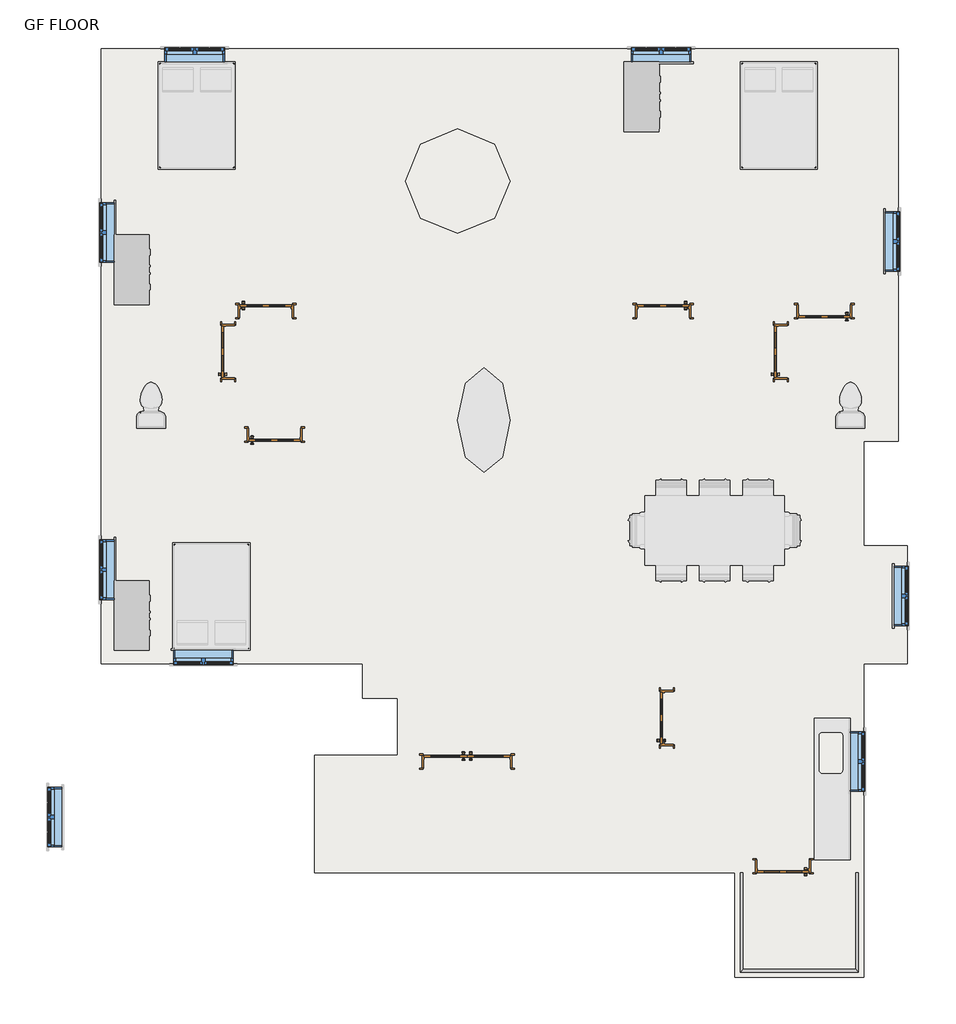
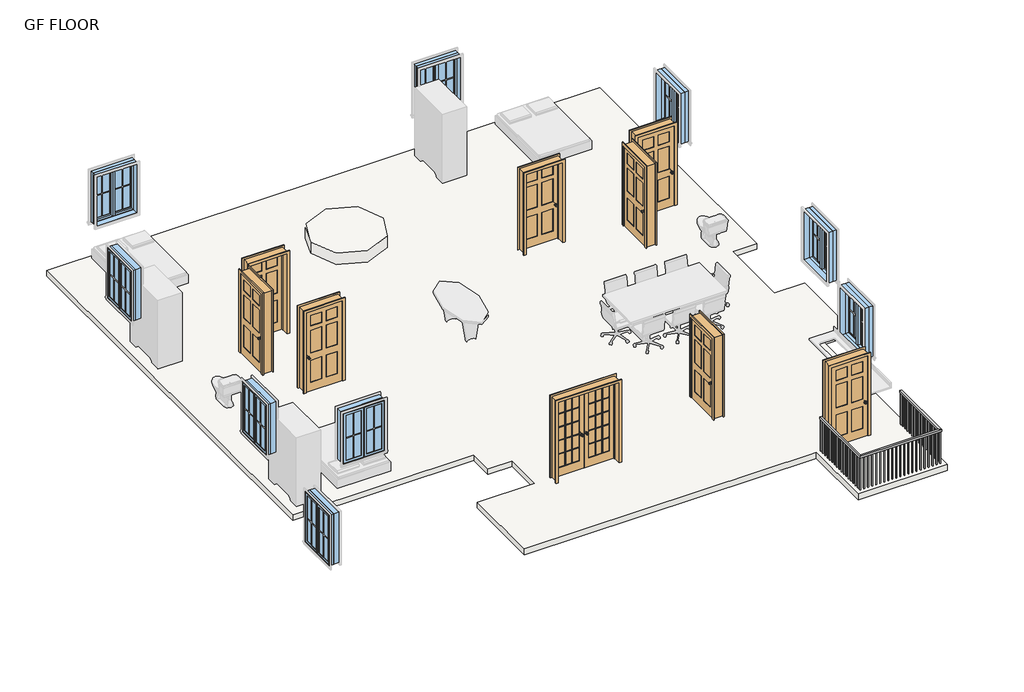
# One storey, part 1 of 2: 9 doors, 9 windows, 2 slabs, 1 railing.
"""IFC4 building model written with IfcOpenShell, lengths in millimetres."""

from ifc_helpers import new_model, si_unit, point, frame, frame_2d, origin, place, context, project, spatial, polyline, circle_curve, trimmed, segment, composite_curve, outline, extrude, faceted_brep, transform, mapped, element, save
from components import door_610bc5f6, door_d86b6c54, door_c5239341, window_c95ebb39

model = new_model("IFC4")

# Units and contexts
model_context = context("Model", 3, world=origin())
ifc_project = project(units=[si_unit("LENGTHUNIT", "METRE", prefix="MILLI")], contexts=[model_context])

# Site, building, storey
site = spatial("IfcSite", under=ifc_project)
building = spatial("IfcBuilding", under=site)
storey = spatial("IfcBuildingStorey", under=building, Name="GF FLOOR", Elevation=914.4)

# Doors
placement = place(None, origin())
door_shape = door_610bc5f6(model_context)
element("IfcDoor", 1, ObjectType="Door-Interior-Double-Full Glass-Wood : 60\" x 84\"", at=placement, inside=storey, context=model_context, shape_type="MappedRepresentation", body=[
    mapped(door_shape, transform((4931.2512825, 2078.7656886, 914.4), x_axis=(1.0, 0.0, 0.0), y_axis=(0.0, 1.0, 0.0), z_axis=(0.0, 0.0, 1.0))),
])
door_2_shape = door_d86b6c54(model_context)
element("IfcDoor", 2, ObjectType="Door-Interior-Single-6_Panel-Wood : 36\" x 84\"", at=placement, inside=storey, context=model_context, shape_type="MappedRepresentation", body=[
    mapped(door_2_shape, transform((8420.5762825, 2837.5906886, 914.4), x_axis=(0.0, 1.0, 0.0), y_axis=(-1.0, 0.0, 0.0), z_axis=(0.0, 0.0, 1.0))),
])
element("IfcDoor", 3, ObjectType="Door-Interior-Single-6_Panel-Wood : 36\" x 84\"", at=placement, inside=storey, context=model_context, shape_type="MappedRepresentation", body=[
    mapped(door_2_shape, transform((10455.7512825, 243.6156886, 914.4), x_axis=(-1.0, 0.0, 0.0), y_axis=(0.0, -1.0, 0.0), z_axis=(0.0, 0.0, 1.0))),
])
element("IfcDoor", 4, ObjectType="Door-Interior-Single-6_Panel-Wood : 36\" x 84\"", at=placement, inside=storey, context=model_context, shape_type="MappedRepresentation", body=[
    mapped(door_2_shape, transform((11179.6512825, 9946.4156886, 914.4), x_axis=(-1.0, 0.0, 0.0), y_axis=(0.0, -1.0, 0.0), z_axis=(0.0, 0.0, 1.0))),
])
element("IfcDoor", 5, ObjectType="Door-Interior-Single-6_Panel-Wood : 36\" x 84\"", at=placement, inside=storey, context=model_context, shape_type="MappedRepresentation", body=[
    mapped(door_2_shape, transform((749.7762825, 9238.3906886, 914.4), x_axis=(0.0, 1.0, 0.0), y_axis=(-1.0, 0.0, 0.0), z_axis=(0.0, 0.0, 1.0))),
])
element("IfcDoor", 6, ObjectType="Door-Interior-Single-6_Panel-Wood : 36\" x 84\"", at=placement, inside=storey, context=model_context, shape_type="MappedRepresentation", body=[
    mapped(door_2_shape, transform((1413.3512825, 9952.7656886, 914.4), x_axis=(1.0, 0.0, 0.0), y_axis=(0.0, 1.0, 0.0), z_axis=(0.0, 0.0, 1.0))),
])
element("IfcDoor", 7, ObjectType="Door-Interior-Single-6_Panel-Wood : 36\" x 84\"", at=placement, inside=storey, context=model_context, shape_type="MappedRepresentation", body=[
    mapped(door_2_shape, transform((10414.4762825, 9238.3906886, 914.4), x_axis=(0.0, 1.0, 0.0), y_axis=(-1.0, 0.0, 0.0), z_axis=(0.0, 0.0, 1.0))),
])
door_3_shape = door_c5239341(model_context)
element("IfcDoor", 8, ObjectType="Door-Interior-Single-6_Panel-Wood : 36\" x 84\"", at=placement, inside=storey, context=model_context, shape_type="MappedRepresentation", body=[
    mapped(door_3_shape, transform((1565.7512825, 7787.4156886, 914.4), x_axis=(1.0, 0.0, 0.0), y_axis=(0.0, 1.0, 0.0), z_axis=(0.0, 0.0, 1.0))),
])
element("IfcDoor", 9, ObjectType="Door-Interior-Single-6_Panel-Wood : 36\" x 84\"", at=placement, inside=storey, context=model_context, shape_type="MappedRepresentation", body=[
    mapped(door_3_shape, transform((8360.2512825, 9952.7656886, 914.4), x_axis=(-1.0, 0.0, 0.0), y_axis=(0.0, -1.0, 0.0), z_axis=(0.0, 0.0, 1.0))),
])

# Railing
element("IfcRailing", 10, ObjectType="Handrail - Rectangular", at=placement, inside=storey, context=model_context, shape_type="SolidModel", body=[
    faceted_brep([(9757.2512825, 132.4906886, 1828.8), (9757.2512825, 132.4906886, 1778.0), (9706.4512825, 132.4906886, 1778.0), (9706.4512825, 132.4906886, 1828.8), (9757.2512825, -1556.6093114, 1828.8), (9757.2512825, -1556.6093114, 1778.0), (9706.4512825, -1607.4093114, 1778.0), (9706.4512825, -1607.4093114, 1828.8), (11725.7512825, -1556.6093114, 1828.8), (11725.7512825, -1556.6093114, 1778.0), (11776.5512825, -1607.4093114, 1778.0), (11776.5512825, -1607.4093114, 1828.8), (11725.7512825, 132.4906886, 1828.8), (11776.5512825, 132.4906886, 1828.8), (11776.5512825, 132.4906886, 1778.0), (11725.7512825, 132.4906886, 1778.0)], [[[0, 1, 2, 3]], [[1, 0, 4, 5]], [[2, 1, 5, 6]], [[3, 2, 6, 7]], [[0, 3, 7, 4]], [[5, 4, 8, 9]], [[6, 5, 9, 10]], [[7, 6, 10, 11]], [[4, 7, 11, 8]], [[12, 13, 14, 15]], [[9, 8, 12, 15]], [[10, 9, 15, 14]], [[11, 10, 14, 13]], [[8, 11, 13, 12]]]),
    extrude(outline(polyline([(11760.6762825, 34.0656886), (11741.6262825, 34.0656886), (11741.6262825, 53.1156886), (11760.6762825, 53.1156886), (11760.6762825, 34.0656886)])), frame((0.0, 0.0, 914.4), z_axis=(0.0, 0.0, 1.0), x_axis=(1.0, 0.0, 0.0)), (0.0, 0.0, 1.0), 863.6),
    extrude(outline(polyline([(11760.6762825, -67.5343114), (11741.6262825, -67.5343114), (11741.6262825, -48.4843114), (11760.6762825, -48.4843114), (11760.6762825, -67.5343114)])), frame((0.0, 0.0, 914.4), z_axis=(0.0, 0.0, 1.0), x_axis=(1.0, 0.0, 0.0)), (0.0, 0.0, 1.0), 863.6),
    extrude(outline(polyline([(11760.6762825, -169.1343114), (11741.6262825, -169.1343114), (11741.6262825, -150.0843114), (11760.6762825, -150.0843114), (11760.6762825, -169.1343114)])), frame((0.0, 0.0, 914.4), z_axis=(0.0, 0.0, 1.0), x_axis=(1.0, 0.0, 0.0)), (0.0, 0.0, 1.0), 863.6),
    extrude(outline(polyline([(11760.6762825, -270.7343114), (11741.6262825, -270.7343114), (11741.6262825, -251.6843114), (11760.6762825, -251.6843114), (11760.6762825, -270.7343114)])), frame((0.0, 0.0, 914.4), z_axis=(0.0, 0.0, 1.0), x_axis=(1.0, 0.0, 0.0)), (0.0, 0.0, 1.0), 863.6),
    extrude(outline(polyline([(11760.6762825, -372.3343114), (11741.6262825, -372.3343114), (11741.6262825, -353.2843114), (11760.6762825, -353.2843114), (11760.6762825, -372.3343114)])), frame((0.0, 0.0, 914.4), z_axis=(0.0, 0.0, 1.0), x_axis=(1.0, 0.0, 0.0)), (0.0, 0.0, 1.0), 863.6),
    extrude(outline(polyline([(11760.6762825, -473.9343114), (11741.6262825, -473.9343114), (11741.6262825, -454.8843114), (11760.6762825, -454.8843114), (11760.6762825, -473.9343114)])), frame((0.0, 0.0, 914.4), z_axis=(0.0, 0.0, 1.0), x_axis=(1.0, 0.0, 0.0)), (0.0, 0.0, 1.0), 863.6),
    extrude(outline(polyline([(11760.6762825, -575.5343114), (11741.6262825, -575.5343114), (11741.6262825, -556.4843114), (11760.6762825, -556.4843114), (11760.6762825, -575.5343114)])), frame((0.0, 0.0, 914.4), z_axis=(0.0, 0.0, 1.0), x_axis=(1.0, 0.0, 0.0)), (0.0, 0.0, 1.0), 863.6),
    extrude(outline(polyline([(11760.6762825, -677.1343114), (11741.6262825, -677.1343114), (11741.6262825, -658.0843114), (11760.6762825, -658.0843114), (11760.6762825, -677.1343114)])), frame((0.0, 0.0, 914.4), z_axis=(0.0, 0.0, 1.0), x_axis=(1.0, 0.0, 0.0)), (0.0, 0.0, 1.0), 863.6),
    extrude(outline(polyline([(11760.6762825, -778.7343114), (11741.6262825, -778.7343114), (11741.6262825, -759.6843114), (11760.6762825, -759.6843114), (11760.6762825, -778.7343114)])), frame((0.0, 0.0, 914.4), z_axis=(0.0, 0.0, 1.0), x_axis=(1.0, 0.0, 0.0)), (0.0, 0.0, 1.0), 863.6),
    extrude(outline(polyline([(11760.6762825, -880.3343114), (11741.6262825, -880.3343114), (11741.6262825, -861.2843114), (11760.6762825, -861.2843114), (11760.6762825, -880.3343114)])), frame((0.0, 0.0, 914.4), z_axis=(0.0, 0.0, 1.0), x_axis=(1.0, 0.0, 0.0)), (0.0, 0.0, 1.0), 863.6),
    extrude(outline(polyline([(11760.6762825, -981.9343114), (11741.6262825, -981.9343114), (11741.6262825, -962.8843114), (11760.6762825, -962.8843114), (11760.6762825, -981.9343114)])), frame((0.0, 0.0, 914.4), z_axis=(0.0, 0.0, 1.0), x_axis=(1.0, 0.0, 0.0)), (0.0, 0.0, 1.0), 863.6),
    extrude(outline(polyline([(11760.6762825, -1083.5343114), (11741.6262825, -1083.5343114), (11741.6262825, -1064.4843114), (11760.6762825, -1064.4843114), (11760.6762825, -1083.5343114)])), frame((0.0, 0.0, 914.4), z_axis=(0.0, 0.0, 1.0), x_axis=(1.0, 0.0, 0.0)), (0.0, 0.0, 1.0), 863.6),
    extrude(outline(polyline([(11760.6762825, -1185.1343114), (11741.6262825, -1185.1343114), (11741.6262825, -1166.0843114), (11760.6762825, -1166.0843114), (11760.6762825, -1185.1343114)])), frame((0.0, 0.0, 914.4), z_axis=(0.0, 0.0, 1.0), x_axis=(1.0, 0.0, 0.0)), (0.0, 0.0, 1.0), 863.6),
    extrude(outline(polyline([(11760.6762825, -1286.7343114), (11741.6262825, -1286.7343114), (11741.6262825, -1267.6843114), (11760.6762825, -1267.6843114), (11760.6762825, -1286.7343114)])), frame((0.0, 0.0, 914.4), z_axis=(0.0, 0.0, 1.0), x_axis=(1.0, 0.0, 0.0)), (0.0, 0.0, 1.0), 863.6),
    extrude(outline(polyline([(11760.6762825, -1388.3343114), (11741.6262825, -1388.3343114), (11741.6262825, -1369.2843114), (11760.6762825, -1369.2843114), (11760.6762825, -1388.3343114)])), frame((0.0, 0.0, 914.4), z_axis=(0.0, 0.0, 1.0), x_axis=(1.0, 0.0, 0.0)), (0.0, 0.0, 1.0), 863.6),
    extrude(outline(polyline([(11760.6762825, -1489.9343114), (11741.6262825, -1489.9343114), (11741.6262825, -1470.8843114), (11760.6762825, -1470.8843114), (11760.6762825, -1489.9343114)])), frame((0.0, 0.0, 914.4), z_axis=(0.0, 0.0, 1.0), x_axis=(1.0, 0.0, 0.0)), (0.0, 0.0, 1.0), 863.6),
    extrude(outline(polyline([(11652.7262825, -1591.5343114), (11652.7262825, -1572.4843114), (11671.7762825, -1572.4843114), (11671.7762825, -1591.5343114), (11652.7262825, -1591.5343114)])), frame((0.0, 0.0, 914.4), z_axis=(0.0, 0.0, 1.0), x_axis=(1.0, 0.0, 0.0)), (0.0, 0.0, 1.0), 863.6),
    extrude(outline(polyline([(11551.1262825, -1591.5343114), (11551.1262825, -1572.4843114), (11570.1762825, -1572.4843114), (11570.1762825, -1591.5343114), (11551.1262825, -1591.5343114)])), frame((0.0, 0.0, 914.4), z_axis=(0.0, 0.0, 1.0), x_axis=(1.0, 0.0, 0.0)), (0.0, 0.0, 1.0), 863.6),
    extrude(outline(polyline([(11449.5262825, -1591.5343114), (11449.5262825, -1572.4843114), (11468.5762825, -1572.4843114), (11468.5762825, -1591.5343114), (11449.5262825, -1591.5343114)])), frame((0.0, 0.0, 914.4), z_axis=(0.0, 0.0, 1.0), x_axis=(1.0, 0.0, 0.0)), (0.0, 0.0, 1.0), 863.6),
    extrude(outline(polyline([(11347.9262825, -1591.5343114), (11347.9262825, -1572.4843114), (11366.9762825, -1572.4843114), (11366.9762825, -1591.5343114), (11347.9262825, -1591.5343114)])), frame((0.0, 0.0, 914.4), z_axis=(0.0, 0.0, 1.0), x_axis=(1.0, 0.0, 0.0)), (0.0, 0.0, 1.0), 863.6),
    extrude(outline(polyline([(11246.3262825, -1591.5343114), (11246.3262825, -1572.4843114), (11265.3762825, -1572.4843114), (11265.3762825, -1591.5343114), (11246.3262825, -1591.5343114)])), frame((0.0, 0.0, 914.4), z_axis=(0.0, 0.0, 1.0), x_axis=(1.0, 0.0, 0.0)), (0.0, 0.0, 1.0), 863.6),
    extrude(outline(polyline([(11144.7262825, -1591.5343114), (11144.7262825, -1572.4843114), (11163.7762825, -1572.4843114), (11163.7762825, -1591.5343114), (11144.7262825, -1591.5343114)])), frame((0.0, 0.0, 914.4), z_axis=(0.0, 0.0, 1.0), x_axis=(1.0, 0.0, 0.0)), (0.0, 0.0, 1.0), 863.6),
    extrude(outline(polyline([(11043.1262825, -1591.5343114), (11043.1262825, -1572.4843114), (11062.1762825, -1572.4843114), (11062.1762825, -1591.5343114), (11043.1262825, -1591.5343114)])), frame((0.0, 0.0, 914.4), z_axis=(0.0, 0.0, 1.0), x_axis=(1.0, 0.0, 0.0)), (0.0, 0.0, 1.0), 863.6),
    extrude(outline(polyline([(10941.5262825, -1591.5343114), (10941.5262825, -1572.4843114), (10960.5762825, -1572.4843114), (10960.5762825, -1591.5343114), (10941.5262825, -1591.5343114)])), frame((0.0, 0.0, 914.4), z_axis=(0.0, 0.0, 1.0), x_axis=(1.0, 0.0, 0.0)), (0.0, 0.0, 1.0), 863.6),
    extrude(outline(polyline([(10839.9262825, -1591.5343114), (10839.9262825, -1572.4843114), (10858.9762825, -1572.4843114), (10858.9762825, -1591.5343114), (10839.9262825, -1591.5343114)])), frame((0.0, 0.0, 914.4), z_axis=(0.0, 0.0, 1.0), x_axis=(1.0, 0.0, 0.0)), (0.0, 0.0, 1.0), 863.6),
    extrude(outline(polyline([(10738.3262825, -1591.5343114), (10738.3262825, -1572.4843114), (10757.3762825, -1572.4843114), (10757.3762825, -1591.5343114), (10738.3262825, -1591.5343114)])), frame((0.0, 0.0, 914.4), z_axis=(0.0, 0.0, 1.0), x_axis=(1.0, 0.0, 0.0)), (0.0, 0.0, 1.0), 863.6),
    extrude(outline(polyline([(10636.7262825, -1591.5343114), (10636.7262825, -1572.4843114), (10655.7762825, -1572.4843114), (10655.7762825, -1591.5343114), (10636.7262825, -1591.5343114)])), frame((0.0, 0.0, 914.4), z_axis=(0.0, 0.0, 1.0), x_axis=(1.0, 0.0, 0.0)), (0.0, 0.0, 1.0), 863.6),
    extrude(outline(polyline([(10535.1262825, -1591.5343114), (10535.1262825, -1572.4843114), (10554.1762825, -1572.4843114), (10554.1762825, -1591.5343114), (10535.1262825, -1591.5343114)])), frame((0.0, 0.0, 914.4), z_axis=(0.0, 0.0, 1.0), x_axis=(1.0, 0.0, 0.0)), (0.0, 0.0, 1.0), 863.6),
    extrude(outline(polyline([(10433.5262825, -1591.5343114), (10433.5262825, -1572.4843114), (10452.5762825, -1572.4843114), (10452.5762825, -1591.5343114), (10433.5262825, -1591.5343114)])), frame((0.0, 0.0, 914.4), z_axis=(0.0, 0.0, 1.0), x_axis=(1.0, 0.0, 0.0)), (0.0, 0.0, 1.0), 863.6),
    extrude(outline(polyline([(10331.9262825, -1591.5343114), (10331.9262825, -1572.4843114), (10350.9762825, -1572.4843114), (10350.9762825, -1591.5343114), (10331.9262825, -1591.5343114)])), frame((0.0, 0.0, 914.4), z_axis=(0.0, 0.0, 1.0), x_axis=(1.0, 0.0, 0.0)), (0.0, 0.0, 1.0), 863.6),
    extrude(outline(polyline([(10230.3262825, -1591.5343114), (10230.3262825, -1572.4843114), (10249.3762825, -1572.4843114), (10249.3762825, -1591.5343114), (10230.3262825, -1591.5343114)])), frame((0.0, 0.0, 914.4), z_axis=(0.0, 0.0, 1.0), x_axis=(1.0, 0.0, 0.0)), (0.0, 0.0, 1.0), 863.6),
    extrude(outline(polyline([(10128.7262825, -1591.5343114), (10128.7262825, -1572.4843114), (10147.7762825, -1572.4843114), (10147.7762825, -1591.5343114), (10128.7262825, -1591.5343114)])), frame((0.0, 0.0, 914.4), z_axis=(0.0, 0.0, 1.0), x_axis=(1.0, 0.0, 0.0)), (0.0, 0.0, 1.0), 863.6),
    extrude(outline(polyline([(10027.1262825, -1591.5343114), (10027.1262825, -1572.4843114), (10046.1762825, -1572.4843114), (10046.1762825, -1591.5343114), (10027.1262825, -1591.5343114)])), frame((0.0, 0.0, 914.4), z_axis=(0.0, 0.0, 1.0), x_axis=(1.0, 0.0, 0.0)), (0.0, 0.0, 1.0), 863.6),
    extrude(outline(polyline([(9925.5262825, -1591.5343114), (9925.5262825, -1572.4843114), (9944.5762825, -1572.4843114), (9944.5762825, -1591.5343114), (9925.5262825, -1591.5343114)])), frame((0.0, 0.0, 914.4), z_axis=(0.0, 0.0, 1.0), x_axis=(1.0, 0.0, 0.0)), (0.0, 0.0, 1.0), 863.6),
    extrude(outline(polyline([(9823.9262825, -1591.5343114), (9823.9262825, -1572.4843114), (9842.9762825, -1572.4843114), (9842.9762825, -1591.5343114), (9823.9262825, -1591.5343114)])), frame((0.0, 0.0, 914.4), z_axis=(0.0, 0.0, 1.0), x_axis=(1.0, 0.0, 0.0)), (0.0, 0.0, 1.0), 863.6),
    extrude(outline(polyline([(9722.3262825, -1483.5843114), (9741.3762825, -1483.5843114), (9741.3762825, -1502.6343114), (9722.3262825, -1502.6343114), (9722.3262825, -1483.5843114)])), frame((0.0, 0.0, 914.4), z_axis=(0.0, 0.0, 1.0), x_axis=(1.0, 0.0, 0.0)), (0.0, 0.0, 1.0), 863.6),
    extrude(outline(polyline([(9722.3262825, -1381.9843114), (9741.3762825, -1381.9843114), (9741.3762825, -1401.0343114), (9722.3262825, -1401.0343114), (9722.3262825, -1381.9843114)])), frame((0.0, 0.0, 914.4), z_axis=(0.0, 0.0, 1.0), x_axis=(1.0, 0.0, 0.0)), (0.0, 0.0, 1.0), 863.6),
    extrude(outline(polyline([(9722.3262825, -1280.3843114), (9741.3762825, -1280.3843114), (9741.3762825, -1299.4343114), (9722.3262825, -1299.4343114), (9722.3262825, -1280.3843114)])), frame((0.0, 0.0, 914.4), z_axis=(0.0, 0.0, 1.0), x_axis=(1.0, 0.0, 0.0)), (0.0, 0.0, 1.0), 863.6),
    extrude(outline(polyline([(9722.3262825, -1178.7843114), (9741.3762825, -1178.7843114), (9741.3762825, -1197.8343114), (9722.3262825, -1197.8343114), (9722.3262825, -1178.7843114)])), frame((0.0, 0.0, 914.4), z_axis=(0.0, 0.0, 1.0), x_axis=(1.0, 0.0, 0.0)), (0.0, 0.0, 1.0), 863.6),
    extrude(outline(polyline([(9722.3262825, -1077.1843114), (9741.3762825, -1077.1843114), (9741.3762825, -1096.2343114), (9722.3262825, -1096.2343114), (9722.3262825, -1077.1843114)])), frame((0.0, 0.0, 914.4), z_axis=(0.0, 0.0, 1.0), x_axis=(1.0, 0.0, 0.0)), (0.0, 0.0, 1.0), 863.6),
    extrude(outline(polyline([(9722.3262825, -975.5843114), (9741.3762825, -975.5843114), (9741.3762825, -994.6343114), (9722.3262825, -994.6343114), (9722.3262825, -975.5843114)])), frame((0.0, 0.0, 914.4), z_axis=(0.0, 0.0, 1.0), x_axis=(1.0, 0.0, 0.0)), (0.0, 0.0, 1.0), 863.6),
    extrude(outline(polyline([(9722.3262825, -873.9843114), (9741.3762825, -873.9843114), (9741.3762825, -893.0343114), (9722.3262825, -893.0343114), (9722.3262825, -873.9843114)])), frame((0.0, 0.0, 914.4), z_axis=(0.0, 0.0, 1.0), x_axis=(1.0, 0.0, 0.0)), (0.0, 0.0, 1.0), 863.6),
    extrude(outline(polyline([(9722.3262825, -772.3843114), (9741.3762825, -772.3843114), (9741.3762825, -791.4343114), (9722.3262825, -791.4343114), (9722.3262825, -772.3843114)])), frame((0.0, 0.0, 914.4), z_axis=(0.0, 0.0, 1.0), x_axis=(1.0, 0.0, 0.0)), (0.0, 0.0, 1.0), 863.6),
    extrude(outline(polyline([(9722.3262825, -670.7843114), (9741.3762825, -670.7843114), (9741.3762825, -689.8343114), (9722.3262825, -689.8343114), (9722.3262825, -670.7843114)])), frame((0.0, 0.0, 914.4), z_axis=(0.0, 0.0, 1.0), x_axis=(1.0, 0.0, 0.0)), (0.0, 0.0, 1.0), 863.6),
    extrude(outline(polyline([(9722.3262825, -569.1843114), (9741.3762825, -569.1843114), (9741.3762825, -588.2343114), (9722.3262825, -588.2343114), (9722.3262825, -569.1843114)])), frame((0.0, 0.0, 914.4), z_axis=(0.0, 0.0, 1.0), x_axis=(1.0, 0.0, 0.0)), (0.0, 0.0, 1.0), 863.6),
    extrude(outline(polyline([(9722.3262825, -467.5843114), (9741.3762825, -467.5843114), (9741.3762825, -486.6343114), (9722.3262825, -486.6343114), (9722.3262825, -467.5843114)])), frame((0.0, 0.0, 914.4), z_axis=(0.0, 0.0, 1.0), x_axis=(1.0, 0.0, 0.0)), (0.0, 0.0, 1.0), 863.6),
    extrude(outline(polyline([(9722.3262825, -365.9843114), (9741.3762825, -365.9843114), (9741.3762825, -385.0343114), (9722.3262825, -385.0343114), (9722.3262825, -365.9843114)])), frame((0.0, 0.0, 914.4), z_axis=(0.0, 0.0, 1.0), x_axis=(1.0, 0.0, 0.0)), (0.0, 0.0, 1.0), 863.6),
    extrude(outline(polyline([(9722.3262825, -264.3843114), (9741.3762825, -264.3843114), (9741.3762825, -283.4343114), (9722.3262825, -283.4343114), (9722.3262825, -264.3843114)])), frame((0.0, 0.0, 914.4), z_axis=(0.0, 0.0, 1.0), x_axis=(1.0, 0.0, 0.0)), (0.0, 0.0, 1.0), 863.6),
    extrude(outline(polyline([(9722.3262825, -162.7843114), (9741.3762825, -162.7843114), (9741.3762825, -181.8343114), (9722.3262825, -181.8343114), (9722.3262825, -162.7843114)])), frame((0.0, 0.0, 914.4), z_axis=(0.0, 0.0, 1.0), x_axis=(1.0, 0.0, 0.0)), (0.0, 0.0, 1.0), 863.6),
    extrude(outline(polyline([(9722.3262825, -61.1843114), (9741.3762825, -61.1843114), (9741.3762825, -80.2343114), (9722.3262825, -80.2343114), (9722.3262825, -61.1843114)])), frame((0.0, 0.0, 914.4), z_axis=(0.0, 0.0, 1.0), x_axis=(1.0, 0.0, 0.0)), (0.0, 0.0, 1.0), 863.6),
    extrude(outline(polyline([(9722.3262825, 40.4156886), (9741.3762825, 40.4156886), (9741.3762825, 21.3656886), (9722.3262825, 21.3656886), (9722.3262825, 40.4156886)])), frame((0.0, 0.0, 914.4), z_axis=(0.0, 0.0, 1.0), x_axis=(1.0, 0.0, 0.0)), (0.0, 0.0, 1.0), 863.6),
    extrude(outline(polyline([(11741.6262825, -1591.5343114), (11741.6262825, -1572.4843114), (11760.6762825, -1572.4843114), (11760.6762825, -1591.5343114), (11741.6262825, -1591.5343114)])), frame((0.0, 0.0, 914.4), z_axis=(0.0, 0.0, 1.0), x_axis=(1.0, 0.0, 0.0)), (0.0, 0.0, 1.0), 863.6),
    extrude(outline(polyline([(9722.3262825, -1572.4843114), (9741.3762825, -1572.4843114), (9741.3762825, -1591.5343114), (9722.3262825, -1591.5343114), (9722.3262825, -1572.4843114)])), frame((0.0, 0.0, 914.4), z_axis=(0.0, 0.0, 1.0), x_axis=(1.0, 0.0, 0.0)), (0.0, 0.0, 1.0), 863.6),
    extrude(outline(polyline([(11760.6762825, 113.4406886), (11741.6262825, 113.4406886), (11741.6262825, 132.4906886), (11760.6762825, 132.4906886), (11760.6762825, 113.4406886)])), frame((0.0, 0.0, 914.4), z_axis=(0.0, 0.0, 1.0), x_axis=(1.0, 0.0, 0.0)), (0.0, 0.0, 1.0), 863.6),
    extrude(outline(polyline([(9722.3262825, 132.4906886), (9741.3762825, 132.4906886), (9741.3762825, 113.4406886), (9722.3262825, 113.4406886), (9722.3262825, 132.4906886)])), frame((0.0, 0.0, 914.4), z_axis=(0.0, 0.0, 1.0), x_axis=(1.0, 0.0, 0.0)), (0.0, 0.0, 1.0), 863.6),
])

# Slabs
element("IfcSlab", 11, at=placement, inside=storey, context=model_context, shape_type="SweptSolid", body=[
    extrude(outline(polyline([(12475.0512825, 14534.2906886), (12475.0512825, 7676.2906886), (11865.4512825, 7676.2906886), (11865.4512825, 5847.4906886), (12627.4512825, 5847.4906886), (12627.4512825, 3790.0906886), (11865.4512825, 3790.0906886), (11865.4512825, -1696.3093114), (9617.5512825, -1696.3093114), (9617.5512825, 132.4906886), (2264.2512825, 132.4906886), (2264.2512825, 2189.8906886), (3712.0512825, 2189.8906886), (3712.0512825, 3180.4906886), (3102.4512825, 3180.4906886), (3102.4512825, 3790.0906886), (-1469.5487175, 3790.0906886), (-1469.5487175, 14534.2906886), (12475.0512825, 14534.2906886)])), frame((0.0, 0.0, 762.0), z_axis=(0.0, 0.0, 1.0), x_axis=(1.0, 0.0, 0.0)), (0.0, 0.0, 1.0), 152.4),
])
element("IfcSlab", 12, at=placement, inside=storey, context=model_context, shape_type="SweptSolid", body=[
    extrude(outline(composite_curve([segment(trimmed(circle_curve(frame_2d((4766.1512825, 12220.6401132)), 914.4), [point((3851.7512825, 12220.6401132))], [point((5680.5512825, 12220.6401132))], False, "CARTESIAN"), True, "CONTINUOUS"), segment(trimmed(circle_curve(frame_2d((4766.1512825, 12220.6401132)), 914.4), [point((5680.5512825, 12220.6401132))], [point((3851.7512825, 12220.6401132))], False, "CARTESIAN"), True, "CONTINUOUS")], self_intersect=False)), frame((0.0, 0.0, 914.4), z_axis=(0.0, 0.0, 1.0), x_axis=(1.0, 0.0, 0.0)), (0.0, 0.0, 1.0), 304.8),
])

# Windows
window_shape = window_c95ebb39(model_context)
element("IfcWindow", 13, ObjectType="Window-Casement-Double : 41\" x 53\"", at=placement, inside=storey, context=model_context, shape_type="MappedRepresentation", body=[
    mapped(window_shape, transform((321.1512825, 3904.3906886, 914.4), x_axis=(-1.0, 0.0, 0.0), y_axis=(0.0, -1.0, 0.0), z_axis=(0.0, 0.0, 1.0))),
])
element("IfcWindow", 14, ObjectType="Window-Casement-Double : 41\" x 53\"", at=placement, inside=storey, context=model_context, shape_type="MappedRepresentation", body=[
    mapped(window_shape, transform((-1355.2487175, 5428.3906886, 914.4), x_axis=(0.0, 1.0, 0.0), y_axis=(-1.0, 0.0, 0.0), z_axis=(0.0, 0.0, 1.0))),
])
element("IfcWindow", 15, ObjectType="Window-Casement-Double : 41\" x 53\"", at=placement, inside=storey, context=model_context, shape_type="MappedRepresentation", body=[
    mapped(window_shape, transform((-1355.2487175, 11321.1906886, 914.4), x_axis=(0.0, 1.0, 0.0), y_axis=(-1.0, 0.0, 0.0), z_axis=(0.0, 0.0, 1.0))),
])
element("IfcWindow", 16, ObjectType="Window-Casement-Double : 41\" x 53\"", at=placement, inside=storey, context=model_context, shape_type="MappedRepresentation", body=[
    mapped(window_shape, transform((168.7512825, 14419.9906886, 914.4), x_axis=(1.0, 0.0, 0.0), y_axis=(0.0, 1.0, 0.0), z_axis=(0.0, 0.0, 1.0))),
])
element("IfcWindow", 17, ObjectType="Window-Casement-Double : 41\" x 53\"", at=placement, inside=storey, context=model_context, shape_type="MappedRepresentation", body=[
    mapped(window_shape, transform((8322.1512825, 14419.9906886, 914.4), x_axis=(1.0, 0.0, 0.0), y_axis=(0.0, 1.0, 0.0), z_axis=(0.0, 0.0, 1.0))),
])
element("IfcWindow", 18, ObjectType="Window-Casement-Double : 41\" x 53\"", at=placement, inside=storey, context=model_context, shape_type="MappedRepresentation", body=[
    mapped(window_shape, transform((12360.7512825, 11168.7906886, 914.4), x_axis=(0.0, -1.0, 0.0), y_axis=(1.0, 0.0, 0.0), z_axis=(0.0, 0.0, 1.0))),
])
element("IfcWindow", 19, ObjectType="Window-Casement-Double : 41\" x 53\"", at=placement, inside=storey, context=model_context, shape_type="MappedRepresentation", body=[
    mapped(window_shape, transform((11751.1512825, 2075.5906886, 914.4), x_axis=(0.0, -1.0, 0.0), y_axis=(1.0, 0.0, 0.0), z_axis=(0.0, 0.0, 1.0))),
])
element("IfcWindow", 20, ObjectType="Window-Casement-Double : 41\" x 53\"", at=placement, inside=storey, context=model_context, shape_type="MappedRepresentation", body=[
    mapped(window_shape, transform((12513.1512825, 4971.1906886, 914.4), x_axis=(0.0, -1.0, 0.0), y_axis=(1.0, 0.0, 0.0), z_axis=(0.0, 0.0, 1.0))),
])
element("IfcWindow", 21, ObjectType="Window-Casement-Double : 41\" x 53\"", at=placement, inside=storey, context=model_context, shape_type="MappedRepresentation", body=[
    mapped(window_shape, transform((-2269.6487175, 1104.0406886, 914.4), x_axis=(0.0, 1.0, 0.0), y_axis=(-1.0, 0.0, 0.0), z_axis=(0.0, 0.0, 1.0))),
])

save(model, "model.ifc")

# Revit data of these elements
# Type "Door-Interior-Double-Full Glass-Wood : 60\" x 84\""
#   Type Mark = "8"
#   Assembly Code = "C1020300"
#   Analytic Construction = "French door, wood frame with single glass"
#   Top Rail = 0' - 4 11/16"
#   Thickness = 0' - 1 3/8"
#   Thermal Resistance (R) = 1.0696 (h·ft²·°F)/BTU
#   Swing Angle [instance default] = 90.00°
#   Stiles = 0' - 4 3/4"
#   Rough Width = 5' - 2"
#   Rough Height = 7' - 1"
#   Panel Width = 2' - 6"
#   Height = 7' - 0"
#   Width = 5' - 0"
#   Heat Transfer Coefficient (U) = 0.9350 BTU/(h·ft²·°F)
#   Bottom Rail = 0' - 9 1/8"
#   Show Grill [instance default] = yes
#   Trim Material = Cherry
#   Panel Material = Cherry
#   Frame Material = Cherry
#   Door Handle Material = Aluminum
#   Visual Light Transmittance = 0
#   Solar Heat Gain Coefficient = 0
#   Wall Closure = (empty or 0)
#   Function = (empty or 0)
# Type "Door-Interior-Single-6_Panel-Wood : 36\" x 84\""
#   Type Mark = "9"
#   Assembly Code = "C1020300"
#   Analytic Construction = "Wooden"
#   Top Rail = 0' - 4 11/16"
#   Top Panel = 0' - 11"
#   Thickness = 0' - 1 3/8"
#   Thermal Resistance (R) = 2.5876 (h·ft²·°F)/BTU
#   Swing Angle [instance default] = 90.00°
#   Stiles = 0' - 4 3/4"
#   Rough Width = 3' - 2"
#   Rough Height = 7' - 1"
#   Mullion = 0' - 4 1/2"
#   Lock Rail = 0' - 7 1/2"
#   Intermediate Rail = 0' - 4 1/2"
#   Height = 7' - 0"
#   Width = 3' - 0"
#   Heat Transfer Coefficient (U) = 0.3865 BTU/(h·ft²·°F)
#   Bottom Rail = 0' - 9 1/8"
#   Trim Material = Cherry
#   Panel Material = Cherry
#   Frame Material = Cherry
#   Door Handle Material = Aluminum
#   Visual Light Transmittance = 0
#   Solar Heat Gain Coefficient = 0
#   Wall Closure = (empty or 0)
#   Function = (empty or 0)
# Type "Handrail - Rectangular"
#   Assembly Code = "C2010400"
#   built-in parameter 1008612 = 0.0416667 (stored number, unit not read)
#   built-in parameter 1008611 = 0.0416667 (stored number, unit not read)
#   built-in parameter 1008609 = 0.333333 (stored number, unit not read)
#   built-in parameter 1008604 = 0.166667 (stored number, unit not read)
#   built-in parameter 1008603 = 0.166667 (stored number, unit not read)
#   Railing Height = 3' - 0"
#   built-in parameter 1008630 = 2
#   built-in parameter 1008610 = 2
#   built-in parameter 1008618 = Baluster - Square : 3/4"
# Type
#   Assembly Code = "B1010"
#   Function = 0
#   Layers, outside or top first: 0' - 6" "Concrete, Cast-in-Place gray" (function 1)
# Type
#   Assembly Code = "B1010"
#   Function = 0
#   Layers, outside or top first: 1' - 0" "Earth" (function 1)
# Type "Window-Casement-Double : 41\" x 53\""
#   Type Mark = "15"
#   Fire Rating = "0.5h"
#   Assembly Code = "B2020100"
#   Analytic Construction = "Double glazing - domestic"
#   Frame Extension [instance default] = 0' - 0 1/4"
#   Window Inset [instance default] = 0' - 0"
#   Wall Thickness [instance default] = 0' - 6"
#   Interior Wall Closure [instance default] = 0' - 2 1/4"
#   Half Width = 1' - 8 1/2"
#   Visual Light Transmittance = 0.81
#   Thermal Resistance (R) = 1.8146 (h·ft²·°F)/BTU
#   Solar Heat Gain Coefficient = 0.76
#   Rough Width = 3' - 5 1/2"
#   Rough Height = 4' - 5 1/2"
#   Height = 4' - 5"
#   Heat Transfer Coefficient (U) = 0.5511 BTU/(h·ft²·°F)
#   Exterior Wall Closure [instance default] = 0' - 1 1/4"
#   Extension Jamb [instance default] = 0' - 2 1/4"
#   Default Sill Height = 3' - 0"
#   Width = 3' - 5"
#   Define Thermal Properties by = 0
#   Muntin Visibility = yes
#   Interior Trim Visibility [instance default] = yes
#   Exterior Trim Visibility [instance default] = yes
#   Extension Jamb Visibility [instance default] = yes
#   Interior Trim Material = Wood - Stained
#   Muntin Pattern = Muntin Pattern_2x2 : Muntin Pattern_2x2
#   Interior Trim = Trim-Window-Interior-Flat : Picture Frame
#   Interior Frame Material = Wood - Stained
#   Glass Panel Material = Glass
#   Exterior Trim Material = Clad - White
#   Exterior Trim = Trim-Window-Exterior-Flat : with Sill
#   Exterior Frame Material = Clad - White
#   Wall Closure = (empty or 0)
# Element 1 (IfcDoor, "Door-Interior-Double-Full Glass-Wood : 60\" x 84\"")
#   Swing Angle = 90.00°
#   Show Grill = yes
#   Phase Created = New Construction
#   Materials on its faces: "Cherry", "Aluminum", "Glass"
# Elements 2, 3, 4, 5, 6, 7, 8, 9 (IfcDoor, "Door-Interior-Single-6_Panel-Wood : 36\" x 84\"")
#   Swing Angle = 90.00°
#   Phase Created = New Construction
#   Materials on its faces: "Cherry", "Aluminum"
# Element 10 (IfcRailing, "Handrail - Rectangular")
#   Phase Created = New Construction
# Element 11 (IfcSlab)
#   Height Offset From Level = 0' - 0"
#   Phase Created = New Construction
#   Materials on its faces: "Concrete, Cast-in-Place gray"
# Element 12 (IfcSlab)
#   Height Offset From Level = 1' - 0"
#   Phase Created = New Construction
#   Materials on its faces: "Earth", "Grass"
# Element 13 (IfcWindow, "Window-Casement-Double : 41\" x 53\"")
#   Mark = "1"
#   Window Inset = 0' - 0"
#   Interior Wall Closure = 0' - 2 1/4"
#   Frame Extension = 0' - 0 1/4"
#   Exterior Wall Closure = 0' - 1 1/4"
#   Interior Trim Visibility = yes
#   Exterior Trim Visibility = yes
#   Phase Created = New Construction
#   Materials on its faces: "Wood - Stained", "Glass", "Clad - White"
# Element 14 (IfcWindow, "Window-Casement-Double : 41\" x 53\"")
#   Mark = "2"
#   Window Inset = 0' - 0"
#   Interior Wall Closure = 0' - 2 1/4"
#   Frame Extension = 0' - 0 1/4"
#   Exterior Wall Closure = 0' - 1 1/4"
#   Interior Trim Visibility = yes
#   Exterior Trim Visibility = yes
#   Phase Created = New Construction
#   Materials on its faces: "Wood - Stained", "Glass", "Clad - White"
# Element 15 (IfcWindow, "Window-Casement-Double : 41\" x 53\"")
#   Mark = "3"
#   Window Inset = 0' - 0"
#   Interior Wall Closure = 0' - 2 1/4"
#   Frame Extension = 0' - 0 1/4"
#   Exterior Wall Closure = 0' - 1 1/4"
#   Interior Trim Visibility = yes
#   Exterior Trim Visibility = yes
#   Phase Created = New Construction
#   Materials on its faces: "Wood - Stained", "Glass", "Clad - White"
# Element 16 (IfcWindow, "Window-Casement-Double : 41\" x 53\"")
#   Mark = "4"
#   Window Inset = 0' - 0"
#   Interior Wall Closure = 0' - 2 1/4"
#   Frame Extension = 0' - 0 1/4"
#   Exterior Wall Closure = 0' - 1 1/4"
#   Interior Trim Visibility = yes
#   Exterior Trim Visibility = yes
#   Phase Created = New Construction
#   Materials on its faces: "Wood - Stained", "Glass", "Clad - White"
# Element 17 (IfcWindow, "Window-Casement-Double : 41\" x 53\"")
#   Mark = "5"
#   Window Inset = 0' - 0"
#   Interior Wall Closure = 0' - 2 1/4"
#   Frame Extension = 0' - 0 1/4"
#   Exterior Wall Closure = 0' - 1 1/4"
#   Interior Trim Visibility = yes
#   Exterior Trim Visibility = yes
#   Phase Created = New Construction
#   Materials on its faces: "Wood - Stained", "Glass", "Clad - White"
# Element 18 (IfcWindow, "Window-Casement-Double : 41\" x 53\"")
#   Mark = "6"
#   Window Inset = 0' - 0"
#   Interior Wall Closure = 0' - 2 1/4"
#   Frame Extension = 0' - 0 1/4"
#   Exterior Wall Closure = 0' - 1 1/4"
#   Interior Trim Visibility = yes
#   Exterior Trim Visibility = yes
#   Phase Created = New Construction
#   Materials on its faces: "Wood - Stained", "Glass", "Clad - White"
# Element 19 (IfcWindow, "Window-Casement-Double : 41\" x 53\"")
#   Mark = "7"
#   Window Inset = 0' - 0"
#   Interior Wall Closure = 0' - 2 1/4"
#   Frame Extension = 0' - 0 1/4"
#   Exterior Wall Closure = 0' - 1 1/4"
#   Interior Trim Visibility = yes
#   Exterior Trim Visibility = yes
#   Phase Created = New Construction
#   Materials on its faces: "Wood - Stained", "Glass", "Clad - White"
# Element 20 (IfcWindow, "Window-Casement-Double : 41\" x 53\"")
#   Mark = "8"
#   Window Inset = 0' - 0"
#   Interior Wall Closure = 0' - 2 1/4"
#   Frame Extension = 0' - 0 1/4"
#   Exterior Wall Closure = 0' - 1 1/4"
#   Interior Trim Visibility = yes
#   Exterior Trim Visibility = yes
#   Phase Created = New Construction
#   Materials on its faces: "Wood - Stained", "Glass", "Clad - White"
# Element 21 (IfcWindow, "Window-Casement-Double : 41\" x 53\"")
#   Mark = "9"
#   Window Inset = 0' - 0"
#   Interior Wall Closure = 0' - 2 1/4"
#   Frame Extension = 0' - 0 1/4"
#   Exterior Wall Closure = 0' - 1 1/4"
#   Interior Trim Visibility = yes
#   Exterior Trim Visibility = yes
#   Phase Created = New Construction
#   Materials on its faces: "Wood - Stained", "Glass", "Clad - White"
# Materials
#   "Cherry": class "Wood", colour RGB 226 177 128, transparency 0, Description = "Prunus Serotina", Cost = 0
#   "Aluminum": class "Metal", colour RGB 247 247 247, transparency 0, Description = "Aluminum 6061", Cost = 0
#   "Concrete, Cast-in-Place gray": class "Concrete", colour RGB 192 192 192, transparency 0, Description = "Cast-in-place concrete", Cost = 0
#   "Earth": class "Generic", colour RGB 97 75 62, transparency 0, Description = "Soil", Cost = 0
#   "Wood - Stained": class "Wood", colour RGB 224 178 126, transparency 0, Cost = 0
#   "Glass": class "Glass", colour RGB 0 128 192, transparency 0.75, Description = "Soda Lime Glass", Cost = 0
#   "Clad - White": class "Wood", colour RGB 242 242 238, transparency 0, Cost = 0
#   "Grass": class "Generic", colour RGB 104 137 66, transparency 0, Description = "Physical material.", Cost = 0
